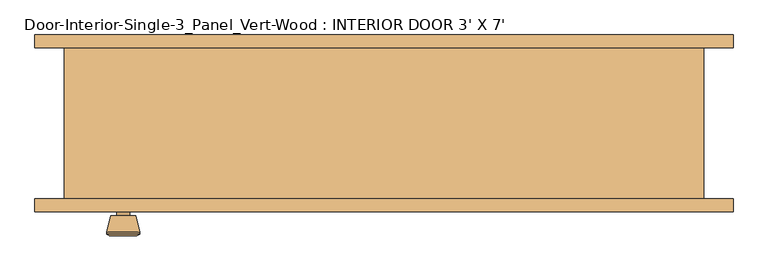
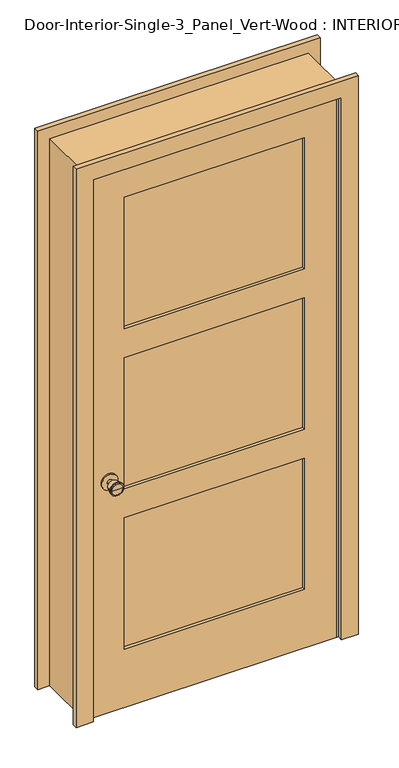
"""IFC4 building model written with IfcOpenShell, lengths in millimetres: door geometry, Door-Interior-Single-3_Panel_Vert-Wood : INTERIOR DOOR 3' X 7'."""

from ifc_helpers import new_model, si_unit, point, frame, frame_2d, origin, place, context, project, spatial, polyline, circle_curve, trimmed, segment, composite_curve, outline, extrude, faceted_brep, source, transform, mapped, element, save
from ifc_brep_helpers import plane_surface, cylinder_surface, revolved_surface, advanced_brep


def door_interior_single_3_panel_vert_wood_interior_door_3_x_7_d98c575a(model_context):
    return source(origin(), model_context, "Body", "SolidModel", [
        advanced_brep(
        [(-393.7, -70.2, 914.4), (-403.7, -70.2, 914.4), (-383.7, -70.2, 914.4), (-373.2241324, -21.2, 914.4), (-414.1758676, -21.2, 914.4), (-393.7, -21.2, 914.4), (-368.7, -23.0278681, 914.4), (-418.7, -23.0278681, 914.4), (-368.7, -26.4915463, 914.4), (-418.7, -26.4915463, 914.4), (-375.063764, -51.2, 914.4), (-412.336236, -51.2, 914.4), (-383.7, -51.2, 914.4), (-403.7, -51.2, 914.4)],
        [
            (0, 1),
            (1, 2, circle_curve(frame((-393.7, -70.2, 914.4), z_axis=(0.0, -1.0, 0.0), x_axis=(-1.0, 0.0, 0.0)), 10.0)),
            (2, 0),
            (2, 1, circle_curve(frame((-393.7, -70.2, 914.4), z_axis=(0.0, -1.0, 0.0), x_axis=(-1.0, 0.0, 0.0)), 10.0)),
            (3, 4, circle_curve(frame((-393.7, -21.2, 914.4), z_axis=(0.0, 1.0, 0.0), x_axis=(-1.0, 0.0, 0.0)), 20.4758676)),
            (4, 5),
            (5, 3),
            (4, 3, circle_curve(frame((-393.7, -21.2, 914.4), z_axis=(0.0, 1.0, 0.0), x_axis=(-1.0, 0.0, 0.0)), 20.4758676)),
            (6, 7, circle_curve(frame((-393.7, -23.0278681, 914.4), z_axis=(0.0, 1.0, 0.0), x_axis=(-1.0, 0.0, 0.0)), 25.0)),
            (7, 4),
            (3, 6),
            (7, 6, circle_curve(frame((-393.7, -23.0278681, 914.4), z_axis=(0.0, 1.0, 0.0), x_axis=(-1.0, 0.0, 0.0)), 25.0)),
            (8, 9, circle_curve(frame((-393.7, -26.4915463, 914.4), z_axis=(0.0, 1.0, 0.0), x_axis=(-1.0, 0.0, 0.0)), 25.0)),
            (9, 7),
            (6, 8),
            (9, 8, circle_curve(frame((-393.7, -26.4915463, 914.4), z_axis=(0.0, 1.0, 0.0), x_axis=(-1.0, 0.0, 0.0)), 25.0)),
            (10, 11, circle_curve(frame((-393.7, -51.2, 914.4), z_axis=(0.0, 1.0, 0.0), x_axis=(-1.0, 0.0, 0.0)), 18.636236)),
            (11, 9),
            (8, 10),
            (11, 10, circle_curve(frame((-393.7, -51.2, 914.4), z_axis=(0.0, 1.0, 0.0), x_axis=(-1.0, 0.0, 0.0)), 18.636236)),
            (12, 13, circle_curve(frame((-393.7, -51.2, 914.4), z_axis=(0.0, 1.0, 0.0), x_axis=(-1.0, 0.0, 0.0)), 10.0)),
            (13, 11),
            (10, 12),
            (13, 12, circle_curve(frame((-393.7, -51.2, 914.4), z_axis=(0.0, 1.0, 0.0), x_axis=(-1.0, 0.0, 0.0)), 10.0)),
            (1, 13),
            (12, 2),
        ],
        [
            plane_surface(frame((-393.7, -70.2, 914.4), z_axis=(0.0, -1.0, 0.0), x_axis=(-1.0, 0.0, 0.0))),
            plane_surface(frame((-393.7, -21.2, 914.4), z_axis=(0.0, 1.0, 0.0), x_axis=(-1.0, 0.0, 0.0))),
            revolved_surface(polyline([(-414.1758676, -21.2, 914.4), (-418.7, -23.0278681, 914.4)]), (-393.7, -70.2, 914.4), (0.0, -1.0, 0.0)),
            cylinder_surface(frame((-393.7, -70.2, 914.4), z_axis=(0.0, -1.0, 0.0), x_axis=(-1.0, 0.0, 0.0)), 25.0),
            revolved_surface(polyline([(-418.7, -26.4915463, 914.4), (-412.336236, -51.2, 914.4)]), (-393.7, -70.2, 914.4), (0.0, -1.0, 0.0)),
            plane_surface(frame((-393.7, -51.2, 914.4), z_axis=(0.0, -1.0, 0.0), x_axis=(-1.0, 0.0, 0.0))),
            cylinder_surface(frame((-393.7, -70.2, 914.4), z_axis=(0.0, -1.0, 0.0), x_axis=(-1.0, 0.0, 0.0)), 10.0),
        ],
        [
            (0, [[1, 2, 3]]),
            (0, [[-3, 4, -1]]),
            (1, [[5, 6, 7]]),
            (1, [[8, -7, -6]]),
            (2, [[9, 10, -5, 11]]),
            (2, [[12, -11, -8, -10]]),
            (3, [[13, 14, -9, 15]]),
            (3, [[16, -15, -12, -14]]),
            (4, [[17, 18, -13, 19]]),
            (4, [[20, -19, -16, -18]]),
            (5, [[21, 22, -17, 23]]),
            (5, [[24, -23, -20, -22]]),
            (6, [[-2, 25, -21, 26]]),
            (6, [[-4, -26, -24, -25]]),
        ],
    ),
        extrude(outline(composite_curve([segment(trimmed(circle_curve(frame_2d((914.4, -393.7)), 30.0), [point((914.4, -423.7))], [point((914.4, -363.7))], False, "CARTESIAN"), True, "CONTINUOUS"), segment(trimmed(circle_curve(frame_2d((914.4, -393.7)), 30.0), [point((914.4, -363.7))], [point((914.4, -423.7))], False, "CARTESIAN"), True, "CONTINUOUS")], self_intersect=False)), frame((0.0, -76.2, 0.0), z_axis=(0.0, 1.0, 0.0), x_axis=(0.0, 0.0, 1.0)), (0.0, 0.0, 1.0), 6.0),
        advanced_brep(
        [(-393.7, -117.125, 914.4), (-383.7, -117.125, 914.4), (-403.7, -117.125, 914.4), (-373.2241324, -166.125, 914.4), (-393.7, -166.125, 914.4), (-414.1758676, -166.125, 914.4), (-368.7, -164.2971319, 914.4), (-418.7, -164.2971319, 914.4), (-368.7, -160.8334537, 914.4), (-418.7, -160.8334537, 914.4), (-375.063764, -136.125, 914.4), (-412.336236, -136.125, 914.4), (-383.7, -136.125, 914.4), (-403.7, -136.125, 914.4)],
        [
            (0, 1),
            (1, 2, circle_curve(frame((-393.7, -117.125, 914.4), z_axis=(0.0, 1.0, 0.0), x_axis=(-1.0, 0.0, 0.0)), 10.0)),
            (2, 0),
            (2, 1, circle_curve(frame((-393.7, -117.125, 914.4), z_axis=(0.0, 1.0, 0.0), x_axis=(-1.0, 0.0, 0.0)), 10.0)),
            (3, 4),
            (4, 5),
            (5, 3, circle_curve(frame((-393.7, -166.125, 914.4), z_axis=(0.0, -1.0, 0.0), x_axis=(-1.0, 0.0, 0.0)), 20.4758676)),
            (3, 5, circle_curve(frame((-393.7, -166.125, 914.4), z_axis=(0.0, -1.0, 0.0), x_axis=(-1.0, 0.0, 0.0)), 20.4758676)),
            (6, 3),
            (5, 7),
            (7, 6, circle_curve(frame((-393.7, -164.2971319, 914.4), z_axis=(0.0, -1.0, 0.0), x_axis=(-1.0, 0.0, 0.0)), 25.0)),
            (6, 7, circle_curve(frame((-393.7, -164.2971319, 914.4), z_axis=(0.0, -1.0, 0.0), x_axis=(-1.0, 0.0, 0.0)), 25.0)),
            (8, 6),
            (7, 9),
            (9, 8, circle_curve(frame((-393.7, -160.8334537, 914.4), z_axis=(0.0, -1.0, 0.0), x_axis=(-1.0, 0.0, 0.0)), 25.0)),
            (8, 9, circle_curve(frame((-393.7, -160.8334537, 914.4), z_axis=(0.0, -1.0, 0.0), x_axis=(-1.0, 0.0, 0.0)), 25.0)),
            (10, 8),
            (9, 11),
            (11, 10, circle_curve(frame((-393.7, -136.125, 914.4), z_axis=(0.0, -1.0, 0.0), x_axis=(-1.0, 0.0, 0.0)), 18.636236)),
            (10, 11, circle_curve(frame((-393.7, -136.125, 914.4), z_axis=(0.0, -1.0, 0.0), x_axis=(-1.0, 0.0, 0.0)), 18.636236)),
            (12, 10),
            (11, 13),
            (13, 12, circle_curve(frame((-393.7, -136.125, 914.4), z_axis=(0.0, -1.0, 0.0), x_axis=(-1.0, 0.0, 0.0)), 10.0)),
            (12, 13, circle_curve(frame((-393.7, -136.125, 914.4), z_axis=(0.0, -1.0, 0.0), x_axis=(-1.0, 0.0, 0.0)), 10.0)),
            (1, 12),
            (13, 2),
        ],
        [
            plane_surface(frame((-393.7, -117.125, 914.4), z_axis=(0.0, 1.0, 0.0), x_axis=(-1.0, 0.0, 0.0))),
            plane_surface(frame((-393.7, -166.125, 914.4), z_axis=(0.0, -1.0, 0.0), x_axis=(-1.0, 0.0, 0.0))),
            revolved_surface(polyline([(-414.1758676, -166.125, 914.4), (-418.7, -164.2971319, 914.4)]), (-393.7, -117.125, 914.4), (0.0, 1.0, 0.0)),
            cylinder_surface(frame((-393.7, -117.125, 914.4), z_axis=(0.0, 1.0, 0.0), x_axis=(-1.0, 0.0, 0.0)), 25.0),
            revolved_surface(polyline([(-418.7, -160.8334537, 914.4), (-412.336236, -136.125, 914.4)]), (-393.7, -117.125, 914.4), (0.0, 1.0, 0.0)),
            plane_surface(frame((-393.7, -136.125, 914.4), z_axis=(0.0, 1.0, 0.0), x_axis=(-1.0, 0.0, 0.0))),
            cylinder_surface(frame((-393.7, -117.125, 914.4), z_axis=(0.0, 1.0, 0.0), x_axis=(-1.0, 0.0, 0.0)), 10.0),
        ],
        [
            (0, [[1, 2, 3]]),
            (0, [[-3, 4, -1]]),
            (1, [[5, 6, 7]]),
            (1, [[-6, -5, 8]]),
            (2, [[9, -7, 10, 11]]),
            (2, [[-10, -8, -9, 12]]),
            (3, [[13, -11, 14, 15]]),
            (3, [[-14, -12, -13, 16]]),
            (4, [[17, -15, 18, 19]]),
            (4, [[-18, -16, -17, 20]]),
            (5, [[21, -19, 22, 23]]),
            (5, [[-22, -20, -21, 24]]),
            (6, [[25, -23, 26, -2]]),
            (6, [[-26, -24, -25, -4]]),
        ],
    ),
        extrude(outline(composite_curve([segment(trimmed(circle_curve(frame_2d((914.4, -393.7)), 30.0), [point((914.4, -423.7))], [point((914.4, -363.7))], False, "CARTESIAN"), True, "CONTINUOUS"), segment(trimmed(circle_curve(frame_2d((914.4, -393.7)), 30.0), [point((914.4, -363.7))], [point((914.4, -423.7))], False, "CARTESIAN"), True, "CONTINUOUS")], self_intersect=False)), frame((0.0, -117.125, 0.0), z_axis=(0.0, 1.0, 0.0), x_axis=(0.0, 0.0, 1.0)), (0.0, 0.0, 1.0), 6.0),
        faceted_brep([(482.6, -111.125, 0.0), (457.2, -111.125, 0.0), (457.2, -76.2, 0.0), (444.5, -76.2, 0.0), (444.5, -41.275, 0.0), (457.2, -41.275, 0.0), (457.2, 117.475, 0.0), (482.6, 117.475, 0.0), (482.6, 117.475, 2159.0), (482.6, -111.125, 2159.0), (457.2, 117.475, 2133.6), (-457.2, 117.475, 2133.6), (-457.2, 117.475, 0.0), (-482.6, 117.475, 0.0), (-482.6, 117.475, 2159.0), (457.2, -41.275, 2133.6), (444.5, -41.275, 2120.9), (-444.5, -41.275, 2120.9), (-444.5, -41.275, 0.0), (-457.2, -41.275, 0.0), (-457.2, -41.275, 2133.6), (444.5, -76.2, 2120.9), (457.2, -76.2, 2133.6), (-457.2, -76.2, 2133.6), (-457.2, -76.2, 0.0), (-444.5, -76.2, 0.0), (-444.5, -76.2, 2120.9), (457.2, -111.125, 2133.6), (-482.6, -111.125, 2159.0), (-482.6, -111.125, 0.0), (-457.2, -111.125, 0.0), (-457.2, -111.125, 2133.6)], [[[0, 1, 2, 3, 4, 5, 6, 7]], [[7, 8, 9, 0]], [[6, 10, 11, 12, 13, 14, 8, 7]], [[5, 15, 10, 6]], [[4, 16, 17, 18, 19, 20, 15, 5]], [[3, 21, 16, 4]], [[2, 22, 23, 24, 25, 26, 21, 3]], [[1, 27, 22, 2]], [[0, 9, 28, 29, 30, 31, 27, 1]], [[8, 14, 28, 9]], [[15, 20, 11, 10]], [[21, 26, 17, 16]], [[27, 31, 23, 22]], [[29, 13, 12, 19, 18, 25, 24, 30]], [[14, 13, 29, 28]], [[20, 19, 12, 11]], [[26, 25, 18, 17]], [[31, 30, 24, 23]]]),
        extrude(outline(polyline([(2133.6, -457.2), (0.0, -457.2), (0.0, 457.2), (2133.6, 457.2), (2133.6, -457.2)]), holes=[polyline([(2014.5375, -336.55), (2014.5375, 336.55), (1496.4833333, 336.55), (1496.4833333, -336.55), (2014.5375, -336.55)]), polyline([(749.8291667, -336.55), (749.8291667, 336.55), (231.775, 336.55), (231.775, -336.55), (749.8291667, -336.55)]), polyline([(1382.1833333, -336.55), (1382.1833333, 336.55), (864.1291667, 336.55), (864.1291667, -336.55), (1382.1833333, -336.55)])]), frame((0.0, -111.125, 0.0), z_axis=(0.0, 1.0, 0.0), x_axis=(0.0, 0.0, 1.0)), (0.0, 0.0, 1.0), 34.925),
        extrude(outline(polyline([(336.55, -87.8416667), (336.55, -99.4833333), (-336.55, -99.4833333), (-336.55, -87.8416667), (336.55, -87.8416667)])), frame((0.0, 0.0, 1496.4833333), z_axis=(0.0, 0.0, 1.0), x_axis=(1.0, 0.0, 0.0)), (0.0, 0.0, 1.0), 518.0541667),
        extrude(outline(polyline([(336.55, -87.8416667), (336.55, -99.4833333), (-336.55, -99.4833333), (-336.55, -87.8416667), (336.55, -87.8416667)])), frame((0.0, 0.0, 231.775), z_axis=(0.0, 0.0, 1.0), x_axis=(1.0, 0.0, 0.0)), (0.0, 0.0, 1.0), 518.0541667),
        extrude(outline(polyline([(336.55, -87.8416667), (336.55, -99.4833333), (-336.55, -99.4833333), (-336.55, -87.8416667), (336.55, -87.8416667)])), frame((0.0, 0.0, 864.1291667), z_axis=(0.0, 0.0, 1.0), x_axis=(1.0, 0.0, 0.0)), (0.0, 0.0, 1.0), 518.0541667),
        extrude(outline(polyline([(0.0, 527.05), (2203.45, 527.05), (2203.45, -527.05), (0.0, -527.05), (0.0, -463.55), (2139.95, -463.55), (2139.95, 463.55), (0.0, 463.55), (0.0, 527.05)])), frame((0.0, -130.175, 0.0), z_axis=(0.0, 1.0, 0.0), x_axis=(0.0, 0.0, 1.0)), (0.0, 0.0, 1.0), 19.05),
        extrude(outline(polyline([(0.0, 527.05), (2203.45, 527.05), (2203.45, -527.05), (0.0, -527.05), (0.0, -463.55), (2139.95, -463.55), (2139.95, 463.55), (0.0, 463.55), (0.0, 527.05)])), frame((0.0, 117.475, 0.0), z_axis=(0.0, 1.0, 0.0), x_axis=(0.0, 0.0, 1.0)), (0.0, 0.0, 1.0), 19.05),
    ])


if __name__ == "__main__":
    model = new_model("IFC4")
    model_context = context("Model", 3, world=origin())
    ifc_project = project(units=[si_unit("LENGTHUNIT", "METRE", prefix="MILLI")], contexts=[model_context])
    site = spatial("IfcSite", under=ifc_project)
    building = spatial("IfcBuilding", under=site)
    placement = place(None, origin())
    door_interior_single_3_panel_vert_wood_interior_door_3_x_7_shape = door_interior_single_3_panel_vert_wood_interior_door_3_x_7_d98c575a(model_context)
    element("IfcDoor", 1, ObjectType="Door-Interior-Single-3_Panel_Vert-Wood : INTERIOR DOOR 3' X 7'", at=placement, inside=building, context=model_context, shape_type="MappedRepresentation", body=[
        mapped(door_interior_single_3_panel_vert_wood_interior_door_3_x_7_shape, transform((0.0, 0.0, 0.0), x_axis=(1.0, 0.0, 0.0), y_axis=(0.0, 1.0, 0.0), z_axis=(0.0, 0.0, 1.0))),
    ])
    save(model, "model.ifc")

# Revit data of these elements
# Type "Door-Interior-Single-3_Panel_Vert-Wood : INTERIOR DOOR 3' X 7'"
#   Type Mark = "10"
#   Assembly Code = "C1020300"
#   Analytic Construction = "Wooden"
#   Top Rail = 0' - 4 11/16"
#   Thickness = 0' - 1 3/8"
#   Thermal Resistance (R) = 2.5876 (h·ft²·°F)/BTU
#   Swing Angle [instance default] = 90.00°
#   Stiles = 0' - 4 3/4"
#   Rough Width = 3' - 2"
#   Rough Height = 7' - 1"
#   Intermediate Rail = 0' - 4 1/2"
#   Height = 7' - 0"
#   Width = 3' - 0"
#   Heat Transfer Coefficient (U) = 0.3865 BTU/(h·ft²·°F)
#   Bottom Rail = 0' - 9 1/8"
#   Trim Material = Cherry
#   Panel Material = Cherry
#   Frame Material = Cherry
#   Door Handle Material = Aluminum
#   Visual Light Transmittance = 0
#   Solar Heat Gain Coefficient = 0
#   Wall Closure = (empty or 0)
#   Function = (empty or 0)
# Element 1 (IfcDoor, "Door-Interior-Single-3_Panel_Vert-Wood : INTERIOR DOOR 3' X 7'")
#   Materials on its faces: "Cherry", "Aluminum"
# Materials
#   "Cherry": class "Wood", colour RGB 226 177 128, transparency 0, Description = "Prunus Serotina", Cost = 0
#   "Aluminum": class "Metal", colour RGB 247 247 247, transparency 0, Description = "Aluminum 6061", Cost = 0
